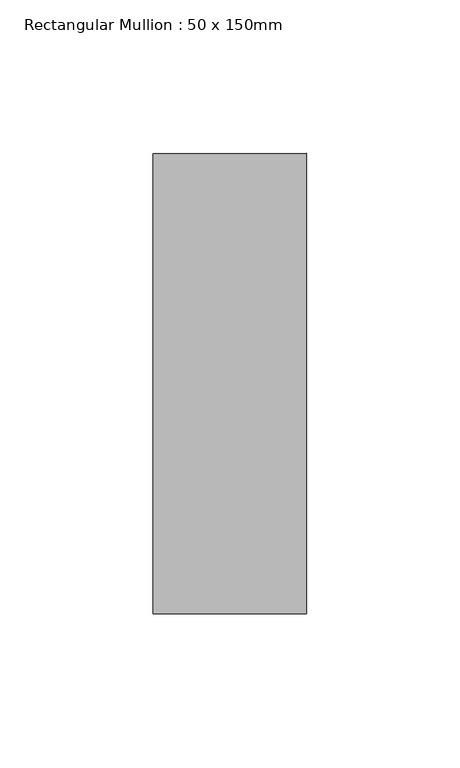
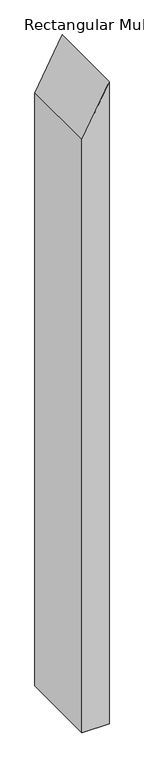
"""IFC4 building model written with IfcOpenShell, lengths in millimetres: member geometry, Rectangular Mullion : 50 x 150mm."""

from ifc_helpers import new_model, si_unit, frame, origin, place, context, project, spatial, polyline, outline, extrude, source, transform, mapped, element, save


def rectangular_mullion_50_x_150mm_dd699d0b(model_context):
    return source(origin(), model_context, "Body", "SweptSolid", [
        extrude(outline(polyline([(0.0, 0.0), (-96.0491063, -50.0), (-1251.2939535, -50.0), (-1251.2939535, 0.0), (0.0, 0.0)])), frame((0.0, -75.0, 0.0), z_axis=(0.0, 1.0, 0.0), x_axis=(0.0, 0.0, 1.0)), (0.0, 0.0, 1.0), 150.0),
    ])


if __name__ == "__main__":
    model = new_model("IFC4")
    model_context = context("Model", 3, world=origin())
    ifc_project = project(units=[si_unit("LENGTHUNIT", "METRE", prefix="MILLI")], contexts=[model_context])
    site = spatial("IfcSite", under=ifc_project)
    building = spatial("IfcBuilding", under=site)
    placement = place(None, origin())
    rectangular_mullion_50_x_150mm_shape = rectangular_mullion_50_x_150mm_dd699d0b(model_context)
    element("IfcMember", 1, ObjectType="Rectangular Mullion : 50 x 150mm", at=placement, inside=building, context=model_context, shape_type="MappedRepresentation", body=[
        mapped(rectangular_mullion_50_x_150mm_shape, transform((0.0, 0.0, 0.0), x_axis=(1.0, 0.0, 0.0), y_axis=(0.0, 1.0, 0.0), z_axis=(0.0, 0.0, 1.0))),
    ])
    save(model, "model.ifc")

# Revit data of these elements
# Type "Rectangular Mullion : 50 x 150mm"
#   built-in parameter 1007304 = 0.492126 (stored number, unit not read)
#   built-in parameter 1007301 = 0.082021 (stored number, unit not read)
#   built-in parameter 1007300 = 0.082021 (stored number, unit not read)
# Element 1 (IfcMember, "Rectangular Mullion : 50 x 150mm")
#   Materials on its faces: "Aluminium"
# Materials
#   "Aluminium": class "Metal", colour RGB 247 247 247, transparency 0, Description = "Aluminium 6061", Cost = 0
